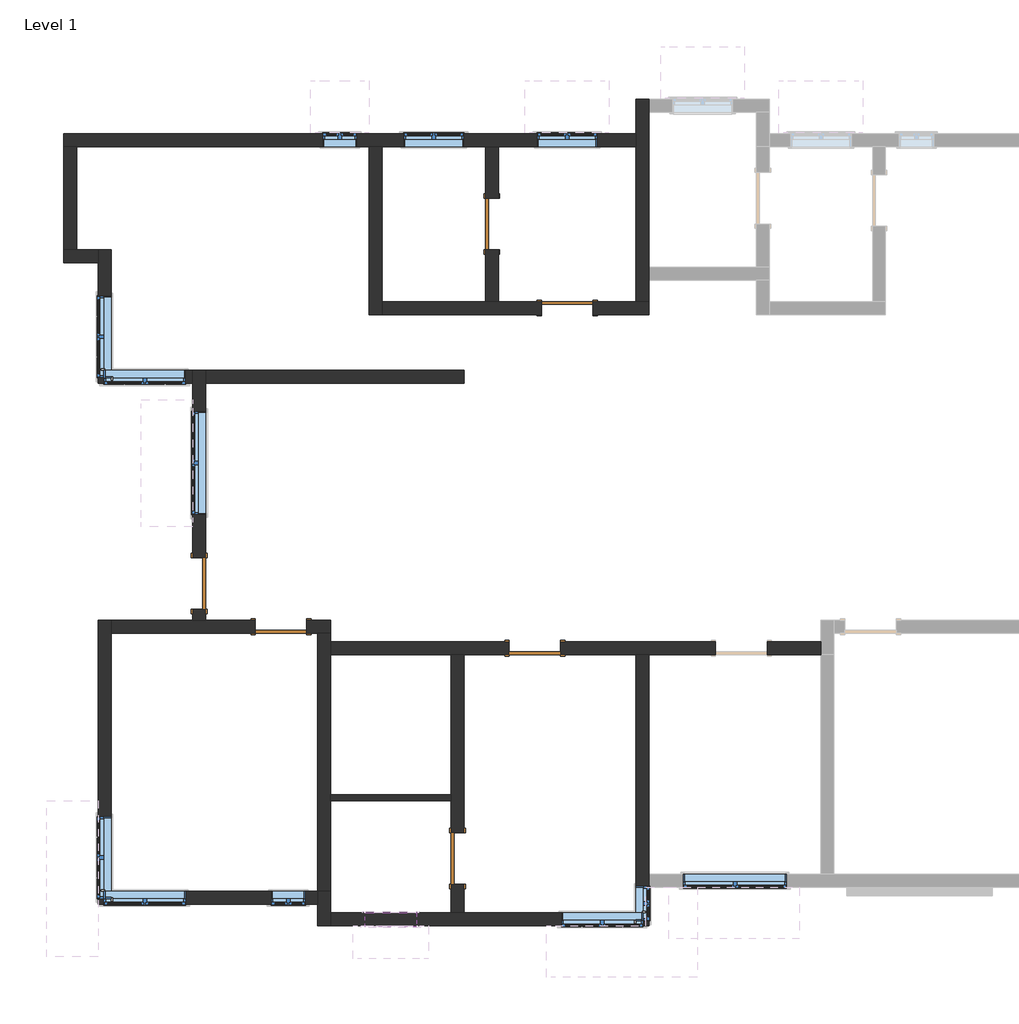
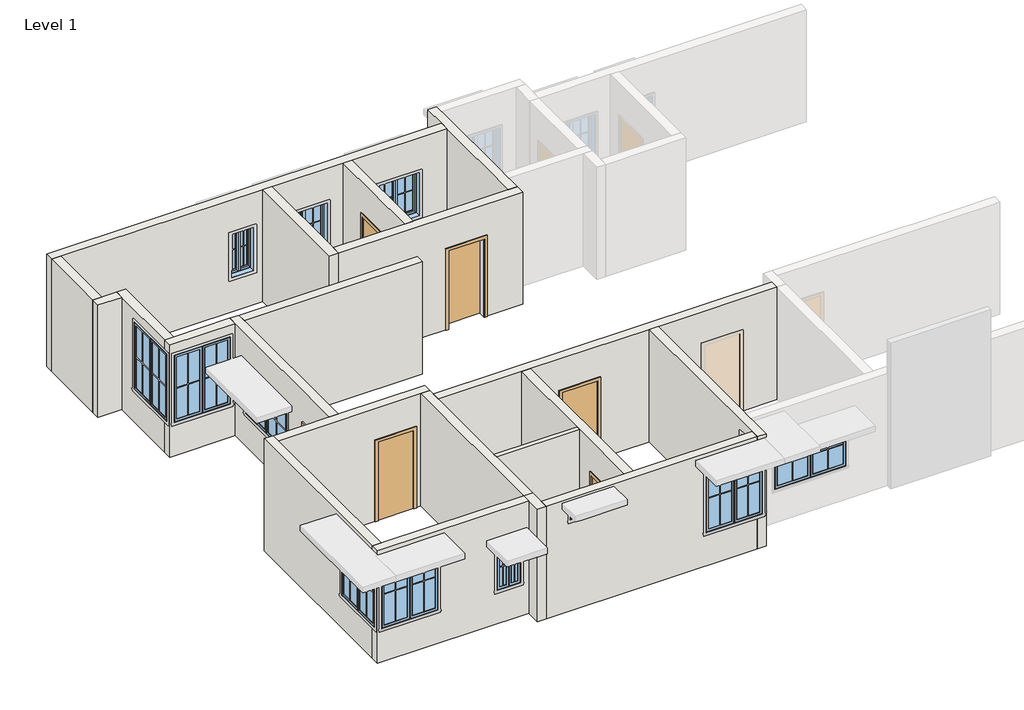
# One storey, part 1 of 3: 21 walls, 13 windows, 6 doors.
"""IFC4 building model written with IfcOpenShell, lengths in millimetres."""

from ifc_helpers import new_model, si_unit, frame, origin, origin_with_axes, place, context, project, spatial, polyline, outline, extrude, faceted_brep, transform, mapped, element, save
from components import door_0ca8825f, door_a90ba1ad, window_0389f97f, window_782a76c6, window_64f85577, window_2032b2cd, window_9ac97e1a, window_bf2f09a8

model = new_model("IFC4")

# Units and contexts
model_context = context("Model", 3, world=origin())
ifc_project = project(units=[si_unit("LENGTHUNIT", "METRE", prefix="MILLI")], contexts=[model_context])

# Site, building, storey
site = spatial("IfcSite", under=ifc_project)
building = spatial("IfcBuilding", under=site)
storey = spatial("IfcBuildingStorey", under=building, Name="Level 1", Elevation=0.0)

# Doors
placement = place(None, origin())
door_shape = door_0ca8825f(model_context)
element("IfcDoor", 1, ObjectType="Single-Flush : 36\" x 84\"", at=placement, inside=storey, context=model_context, shape_type="MappedRepresentation", body=[
    mapped(door_shape, transform((-40282.9145004, 11700.8256148, 0.0), x_axis=(0.0, -1.0, 0.0), y_axis=(1.0, 0.0, 0.0), z_axis=(0.0, 0.0, 1.0))),
])
element("IfcDoor", 2, ObjectType="Single-Flush : 36\" x 84\"", at=placement, inside=storey, context=model_context, shape_type="MappedRepresentation", body=[
    mapped(door_shape, transform((-33767.8145004, 16577.6256148, 0.0), x_axis=(1.0, 0.0, 0.0), y_axis=(0.0, 1.0, 0.0), z_axis=(0.0, 0.0, 1.0))),
])
element("IfcDoor", 3, ObjectType="Single-Flush : 36\" x 84\"", at=placement, inside=storey, context=model_context, shape_type="MappedRepresentation", body=[
    mapped(door_shape, transform((-35101.3145004, 18063.5256148, 0.0), x_axis=(0.0, 1.0, 0.0), y_axis=(-1.0, 0.0, 0.0), z_axis=(0.0, 0.0, 1.0))),
])
element("IfcDoor", 4, ObjectType="Single-Flush : 36\" x 84\"", at=placement, inside=storey, context=model_context, shape_type="MappedRepresentation", body=[
    mapped(door_shape, transform((-34339.3145004, 10557.8256148, 0.0), x_axis=(-1.0, 0.0, 0.0), y_axis=(0.0, -1.0, 0.0), z_axis=(0.0, 0.0, 1.0))),
])
element("IfcDoor", 5, ObjectType="Single-Flush : 36\" x 84\"", at=placement, inside=storey, context=model_context, shape_type="MappedRepresentation", body=[
    mapped(door_shape, transform((-35710.9145004, 6833.4722085, 0.0), x_axis=(0.0, 1.0, 0.0), y_axis=(-1.0, 0.0, 0.0), z_axis=(0.0, 0.0, 1.0))),
])
door_2_shape = door_a90ba1ad(model_context)
element("IfcDoor", 6, ObjectType="Single-Flush : 36\" x 84\"", at=placement, inside=storey, context=model_context, shape_type="MappedRepresentation", body=[
    mapped(door_2_shape, transform((-38835.1145004, 10938.8256148, 0.0), x_axis=(1.0, 0.0, 0.0), y_axis=(0.0, 1.0, 0.0), z_axis=(0.0, 0.0, 1.0))),
])

# Walls
element("IfcWall", 7, ObjectType="wall 4.5", at=placement, inside=storey, context=model_context, shape_type="SweptSolid", body=[
    extrude(outline(polyline([(-35825.2145004, 7852.6472085), (-37958.8145004, 7852.6472085), (-37958.8145004, 7966.9472085), (-35825.2145004, 7966.9472085), (-35825.2145004, 7852.6472085)])), origin_with_axes(), (0.0, 0.0, 1.0), 3048.0),
])
element("IfcWall", 8, ObjectType="wall 9\"", at=placement, inside=storey, context=model_context, shape_type="Brep", body=[
    faceted_brep([(-42683.2145004, 19435.1256148, 0.0), (-42454.6145004, 19435.1256148, 0.0), (-37273.0145004, 19435.1256148, 0.0), (-37044.4145004, 19435.1256148, 0.0), (-35215.6145004, 19435.1256148, 0.0), (-34987.0145004, 19435.1256148, 0.0), (-32548.6145004, 19435.1256148, 0.0), (-32548.6145004, 19435.1256148, 3048.0), (-34987.0145004, 19435.1256148, 3048.0), (-35215.6145004, 19435.1256148, 3048.0), (-37044.4145004, 19435.1256148, 3048.0), (-37273.0145004, 19435.1256148, 3048.0), (-42454.6145004, 19435.1256148, 3048.0), (-42683.2145004, 19435.1256148, 3048.0), (-35596.6145004, 19435.1256148, 2133.6), (-35596.6145004, 19435.1256148, 914.4), (-36663.4145004, 19435.1256148, 914.4), (-36663.4145004, 19435.1256148, 2133.6), (-33234.4145004, 19435.1256148, 2133.6), (-33234.4145004, 19435.1256148, 914.4), (-34301.2145004, 19435.1256148, 914.4), (-34301.2145004, 19435.1256148, 2133.6), (-37488.9145004, 19435.1256148, 2133.6), (-37488.9145004, 19435.1256148, 914.4), (-38098.5145004, 19435.1256148, 914.4), (-38098.5145004, 19435.1256148, 2133.6), (-42683.2145004, 19663.7256148, 0.0), (-42683.2145004, 19663.7256148, 3048.0), (-32548.6145004, 19663.7256148, 3048.0), (-32548.6145004, 19663.7256148, 0.0), (-35596.6145004, 19663.7256148, 2133.6), (-36663.4145004, 19663.7256148, 2133.6), (-36663.4145004, 19663.7256148, 914.4), (-35596.6145004, 19663.7256148, 914.4), (-33234.4145004, 19663.7256148, 2133.6), (-34301.2145004, 19663.7256148, 2133.6), (-34301.2145004, 19663.7256148, 914.4), (-33234.4145004, 19663.7256148, 914.4), (-37488.9145004, 19663.7256148, 2133.6), (-38098.5145004, 19663.7256148, 2133.6), (-38098.5145004, 19663.7256148, 914.4), (-37488.9145004, 19663.7256148, 914.4)], [[[0, 1, 2, 3, 4, 5, 6, 7, 8, 9, 10, 11, 12, 13], [14, 15, 16, 17], [18, 19, 20, 21], [22, 23, 24, 25]], [[26, 27, 28, 29], [30, 31, 32, 33], [34, 35, 36, 37], [38, 39, 40, 41]], [[6, 5, 4, 3, 2, 1, 0, 26, 29]], [[13, 12, 11, 10, 9, 8, 7, 28, 27]], [[7, 6, 29, 28]], [[0, 13, 27, 26]], [[15, 14, 30, 33]], [[16, 15, 33, 32]], [[17, 16, 32, 31]], [[14, 17, 31, 30]], [[19, 18, 34, 37]], [[20, 19, 37, 36]], [[21, 20, 36, 35]], [[18, 21, 35, 34]], [[23, 22, 38, 41]], [[24, 23, 41, 40]], [[25, 24, 40, 39]], [[22, 25, 39, 38]]]),
])
element("IfcWall", 9, ObjectType="wall 9\"", at=placement, inside=storey, context=model_context, shape_type="Brep", body=[
    faceted_brep([(-32320.0145004, 16691.9256148, 0.0), (-32320.0145004, 17072.9256148, 0.0), (-32320.0145004, 17301.5256148, 0.0), (-32320.0145004, 20044.7256148, 0.0), (-32320.0145004, 20273.3256148, 0.0), (-32320.0145004, 20273.3256148, 3048.0), (-32320.0145004, 20044.7256148, 3048.0), (-32320.0145004, 17301.5256148, 3048.0), (-32320.0145004, 17072.9256148, 3048.0), (-32320.0145004, 16691.9256148, 3048.0), (-32548.6145004, 16691.9256148, 0.0), (-32548.6145004, 16691.9256148, 3048.0), (-32548.6145004, 19435.1256148, 3048.0), (-32548.6145004, 19663.7256148, 3048.0), (-32548.6145004, 20273.3256148, 3048.0), (-32548.6145004, 20273.3256148, 0.0), (-32548.6145004, 19663.7256148, 0.0), (-32548.6145004, 19435.1256148, 0.0)], [[[0, 1, 2, 3, 4, 5, 6, 7, 8, 9]], [[10, 11, 12, 13, 14, 15, 16, 17]], [[4, 3, 2, 1, 0, 10, 17, 16, 15]], [[9, 8, 7, 6, 5, 14, 13, 12, 11]], [[5, 4, 15, 14]], [[0, 9, 11, 10]]]),
])
element("IfcWall", 10, ObjectType="wall 9\"", at=placement, inside=storey, context=model_context, shape_type="Brep", body=[
    faceted_brep([(-32548.6145004, 10443.5256148, 0.0), (-32548.6145004, 5871.4472085, 0.0), (-32548.6145004, 5642.8472085, 0.0), (-32548.6145004, 5642.8472085, 914.4), (-32548.6145004, 5871.4472085, 914.4), (-32548.6145004, 6341.3472085, 914.4), (-32548.6145004, 6341.3472085, 2743.2), (-32548.6145004, 5871.4472085, 2743.2), (-32548.6145004, 5642.8472085, 2743.2), (-32548.6145004, 5642.8472085, 3048.0), (-32548.6145004, 5871.4472085, 3048.0), (-32548.6145004, 10443.5256148, 3048.0), (-32320.0145004, 5642.8472085, 0.0), (-32320.0145004, 6328.7256148, 0.0), (-32320.0145004, 6557.3256148, 0.0), (-32320.0145004, 10443.5256148, 0.0), (-32320.0145004, 10443.5256148, 3048.0), (-32320.0145004, 6557.3256148, 3048.0), (-32320.0145004, 6328.7256148, 3048.0), (-32320.0145004, 5642.8472085, 3048.0), (-32320.0145004, 5731.7472085, 914.4), (-32320.0145004, 5731.7472085, 2743.2), (-32320.0145004, 6341.3472085, 2743.2), (-32320.0145004, 6341.3472085, 914.4), (-32421.6145004, 5642.8472085, 2743.2), (-32421.6145004, 5642.8472085, 914.4), (-32421.6145004, 5731.7472085, 914.4), (-32421.6145004, 5731.7472085, 2743.2)], [[[0, 1, 2, 3, 4, 5, 6, 7, 8, 9, 10, 11]], [[12, 13, 14, 15, 16, 17, 18, 19], [20, 21, 22, 23]], [[2, 1, 0, 15, 14, 13, 12]], [[11, 10, 9, 19, 18, 17, 16]], [[2, 12, 19, 9, 8, 24, 25, 3]], [[0, 11, 16, 15]], [[3, 25, 26, 20, 23, 5, 4]], [[25, 24, 27, 26]], [[24, 8, 7, 6, 22, 21, 27]], [[27, 21, 20, 26]], [[5, 23, 22, 6]]]),
])
element("IfcWall", 11, ObjectType="wall 9\"", at=placement, inside=storey, context=model_context, shape_type="Brep", body=[
    faceted_brep([(-32548.6145004, 5871.4472085, 0.0), (-35596.6145004, 5871.4472085, 0.0), (-35825.2145004, 5871.4472085, 0.0), (-37958.8145004, 5871.4472085, 0.0), (-37958.8145004, 5871.4472085, 3048.0), (-35825.2145004, 5871.4472085, 3048.0), (-35596.6145004, 5871.4472085, 3048.0), (-32548.6145004, 5871.4472085, 3048.0), (-32548.6145004, 5871.4472085, 2743.2), (-33869.4145004, 5871.4472085, 2743.2), (-33869.4145004, 5871.4472085, 914.4), (-32548.6145004, 5871.4472085, 914.4), (-37349.2145004, 5871.4472085, 2781.3), (-37349.2145004, 5871.4472085, 2476.5), (-36434.8145004, 5871.4472085, 2476.5), (-36434.8145004, 5871.4472085, 2781.3), (-37958.8145004, 5642.8472085, 0.0), (-32548.6145004, 5642.8472085, 0.0), (-32548.6145004, 5642.8472085, 914.4), (-33869.4145004, 5642.8472085, 914.4), (-33869.4145004, 5642.8472085, 2743.2), (-32548.6145004, 5642.8472085, 2743.2), (-32548.6145004, 5642.8472085, 3048.0), (-37958.8145004, 5642.8472085, 3048.0), (-37349.2145004, 5642.8472085, 2781.3), (-36434.8145004, 5642.8472085, 2781.3), (-36434.8145004, 5642.8472085, 2476.5), (-37349.2145004, 5642.8472085, 2476.5)], [[[0, 1, 2, 3, 4, 5, 6, 7, 8, 9, 10, 11], [12, 13, 14, 15]], [[16, 17, 18, 19, 20, 21, 22, 23], [24, 25, 26, 27]], [[3, 2, 1, 0, 17, 16]], [[7, 6, 5, 4, 23, 22]], [[7, 22, 21, 8]], [[17, 0, 11, 18]], [[4, 3, 16, 23]], [[13, 12, 24, 27]], [[14, 13, 27, 26]], [[15, 14, 26, 25]], [[12, 15, 25, 24]], [[9, 20, 19, 10]], [[10, 19, 18, 11]], [[20, 9, 8, 21]]]),
])
element("IfcWall", 12, ObjectType="wall 9\"", at=placement, inside=storey, context=model_context, shape_type="Brep", body=[
    faceted_brep([(-37958.8145004, 5642.8472085, 0.0), (-37958.8145004, 5871.4472085, 0.0), (-37958.8145004, 6252.5256148, 0.0), (-37958.8145004, 6252.5256148, 3048.0), (-37958.8145004, 5871.4472085, 3048.0), (-37958.8145004, 5642.8472085, 3048.0), (-38187.4145004, 5642.8472085, 0.0), (-38187.4145004, 5642.8472085, 3048.0), (-38187.4145004, 6023.9256148, 3048.0), (-38187.4145004, 6252.5256148, 3048.0), (-38187.4145004, 6252.5256148, 0.0), (-38187.4145004, 6023.9256148, 0.0)], [[[0, 1, 2, 3, 4, 5]], [[6, 7, 8, 9, 10, 11]], [[2, 1, 0, 6, 11, 10]], [[5, 4, 3, 9, 8, 7]], [[0, 5, 7, 6]], [[3, 2, 10, 9]]]),
])
element("IfcWall", 13, ObjectType="wall 9\"", at=placement, inside=storey, context=model_context, shape_type="Brep", body=[
    faceted_brep([(-38187.4145004, 6252.5256148, 0.0), (-41845.0145004, 6252.5256148, 0.0), (-42073.6145004, 6252.5256148, 0.0), (-42073.6145004, 6252.5256148, 914.4), (-41845.0145004, 6252.5256148, 914.4), (-40524.2145004, 6252.5256148, 914.4), (-40524.2145004, 6252.5256148, 2743.2), (-41845.0145004, 6252.5256148, 2743.2), (-42073.6145004, 6252.5256148, 2743.2), (-42073.6145004, 6252.5256148, 3048.0), (-41845.0145004, 6252.5256148, 3048.0), (-38187.4145004, 6252.5256148, 3048.0), (-39012.9145004, 6252.5256148, 2133.6), (-39012.9145004, 6252.5256148, 914.4), (-38403.3145004, 6252.5256148, 914.4), (-38403.3145004, 6252.5256148, 2133.6), (-42073.6145004, 6023.9256148, 0.0), (-38187.4145004, 6023.9256148, 0.0), (-38187.4145004, 6023.9256148, 3048.0), (-42073.6145004, 6023.9256148, 3048.0), (-39012.9145004, 6023.9256148, 914.4), (-39012.9145004, 6023.9256148, 2133.6), (-38403.3145004, 6023.9256148, 2133.6), (-38403.3145004, 6023.9256148, 914.4), (-41972.0145004, 6023.9256148, 914.4), (-41972.0145004, 6023.9256148, 2743.2), (-40524.2145004, 6023.9256148, 2743.2), (-40524.2145004, 6023.9256148, 914.4), (-42073.6145004, 6125.5256148, 2743.2), (-42073.6145004, 6125.5256148, 914.4), (-41972.0145004, 6125.5256148, 914.4), (-41972.0145004, 6125.5256148, 2743.2)], [[[0, 1, 2, 3, 4, 5, 6, 7, 8, 9, 10, 11], [12, 13, 14, 15]], [[16, 17, 18, 19], [20, 21, 22, 23], [24, 25, 26, 27]], [[2, 1, 0, 17, 16]], [[11, 10, 9, 19, 18]], [[0, 11, 18, 17]], [[2, 16, 19, 9, 8, 28, 29, 3]], [[13, 12, 21, 20]], [[14, 13, 20, 23]], [[15, 14, 23, 22]], [[12, 15, 22, 21]], [[25, 24, 30, 31]], [[24, 27, 5, 4, 3, 29, 30]], [[6, 5, 27, 26]], [[26, 25, 31, 28, 8, 7, 6]], [[28, 31, 30, 29]]]),
])
element("IfcWall", 14, ObjectType="wall 9\"", at=placement, inside=storey, context=model_context, shape_type="Brep", body=[
    faceted_brep([(-41845.0145004, 6252.5256148, 0.0), (-41845.0145004, 10824.5256148, 0.0), (-41845.0145004, 11053.1256148, 0.0), (-41845.0145004, 11053.1256148, 3048.0), (-41845.0145004, 10824.5256148, 3048.0), (-41845.0145004, 6252.5256148, 3048.0), (-41845.0145004, 6252.5256148, 2743.2), (-41845.0145004, 7573.3256148, 2743.2), (-41845.0145004, 7573.3256148, 914.4), (-41845.0145004, 6252.5256148, 914.4), (-42073.6145004, 11053.1256148, 0.0), (-42073.6145004, 6252.5256148, 0.0), (-42073.6145004, 6252.5256148, 914.4), (-42073.6145004, 7573.3256148, 914.4), (-42073.6145004, 7573.3256148, 2743.2), (-42073.6145004, 6252.5256148, 2743.2), (-42073.6145004, 6252.5256148, 3048.0), (-42073.6145004, 11053.1256148, 3048.0), (-41972.0145004, 6252.5256148, 2743.2), (-41972.0145004, 6252.5256148, 914.4)], [[[0, 1, 2, 3, 4, 5, 6, 7, 8, 9]], [[10, 11, 12, 13, 14, 15, 16, 17]], [[2, 1, 0, 11, 10]], [[5, 4, 3, 17, 16]], [[5, 16, 15, 18, 6]], [[11, 0, 9, 19, 12]], [[3, 2, 10, 17]], [[7, 14, 13, 8]], [[8, 13, 12, 19, 9]], [[14, 7, 6, 18, 15]]]),
])
element("IfcWall", 15, ObjectType="wall 9\"", at=placement, inside=storey, context=model_context, shape_type="Brep", body=[
    faceted_brep([(-38377.9145004, 10824.5256148, 2133.6), (-38377.9145004, 10824.5256148, 0.0), (-38187.4145004, 10824.5256148, 0.0), (-37958.8145004, 10824.5256148, 0.0), (-37958.8145004, 10824.5256148, 3048.0), (-38187.4145004, 10824.5256148, 3048.0), (-41845.0145004, 10824.5256148, 3048.0), (-41845.0145004, 10824.5256148, 0.0), (-39292.3145004, 10824.5256148, 0.0), (-39292.3145004, 10824.5256148, 2133.6), (-37958.8145004, 11053.1256148, 0.0), (-38377.9145004, 11053.1256148, 0.0), (-38377.9145004, 11053.1256148, 2133.6), (-39292.3145004, 11053.1256148, 2133.6), (-39292.3145004, 11053.1256148, 0.0), (-40168.6145004, 11053.1256148, 0.0), (-40397.2145004, 11053.1256148, 0.0), (-41845.0145004, 11053.1256148, 0.0), (-41845.0145004, 11053.1256148, 3048.0), (-40397.2145004, 11053.1256148, 3048.0), (-40168.6145004, 11053.1256148, 3048.0), (-37958.8145004, 11053.1256148, 3048.0)], [[[0, 1, 2, 3, 4, 5, 6, 7, 8, 9]], [[10, 11, 12, 13, 14, 15, 16, 17, 18, 19, 20, 21]], [[8, 7, 17, 16, 15, 14]], [[3, 2, 1, 11, 10]], [[6, 5, 4, 21, 20, 19, 18]], [[7, 6, 18, 17]], [[4, 3, 10, 21]], [[12, 11, 1, 0]], [[13, 12, 0, 9]], [[14, 13, 9, 8]]]),
])
element("IfcWall", 16, ObjectType="wall 9\"", at=placement, inside=storey, context=model_context, shape_type="Brep", body=[
    faceted_brep([(-40168.6145004, 11053.1256148, 0.0), (-40168.6145004, 11243.6256148, 0.0), (-40168.6145004, 11243.6256148, 2133.6), (-40168.6145004, 12158.0256148, 2133.6), (-40168.6145004, 12158.0256148, 0.0), (-40168.6145004, 15244.1256148, 0.0), (-40168.6145004, 15472.7256148, 0.0), (-40168.6145004, 15472.7256148, 3048.0), (-40168.6145004, 15244.1256148, 3048.0), (-40168.6145004, 11053.1256148, 3048.0), (-40168.6145004, 14748.8256148, 2133.6), (-40168.6145004, 14748.8256148, 914.4), (-40168.6145004, 12920.0256148, 914.4), (-40168.6145004, 12920.0256148, 2133.6), (-40397.2145004, 11243.6256148, 2133.6), (-40397.2145004, 11243.6256148, 0.0), (-40397.2145004, 11053.1256148, 0.0), (-40397.2145004, 11053.1256148, 3048.0), (-40397.2145004, 15244.1256148, 3048.0), (-40397.2145004, 15472.7256148, 3048.0), (-40397.2145004, 15472.7256148, 0.0), (-40397.2145004, 15244.1256148, 0.0), (-40397.2145004, 12158.0256148, 0.0), (-40397.2145004, 12158.0256148, 2133.6), (-40397.2145004, 14748.8256148, 2133.6), (-40397.2145004, 12920.0256148, 2133.6), (-40397.2145004, 12920.0256148, 914.4), (-40397.2145004, 14748.8256148, 914.4)], [[[0, 1, 2, 3, 4, 5, 6, 7, 8, 9], [10, 11, 12, 13]], [[14, 15, 16, 17, 18, 19, 20, 21, 22, 23], [24, 25, 26, 27]], [[16, 15, 1, 0]], [[22, 21, 20, 6, 5, 4]], [[9, 8, 7, 19, 18, 17]], [[0, 9, 17, 16]], [[7, 6, 20, 19]], [[2, 1, 15, 14]], [[3, 2, 14, 23]], [[4, 3, 23, 22]], [[11, 10, 24, 27]], [[12, 11, 27, 26]], [[13, 12, 26, 25]], [[10, 13, 25, 24]]]),
])
element("IfcWall", 17, ObjectType="wall 9\"", at=placement, inside=storey, context=model_context, shape_type="Brep", body=[
    faceted_brep([(-40397.2145004, 15472.7256148, 0.0), (-41845.0145004, 15472.7256148, 0.0), (-42073.6145004, 15472.7256148, 0.0), (-42073.6145004, 15472.7256148, 914.4), (-41845.0145004, 15472.7256148, 914.4), (-40524.2145004, 15472.7256148, 914.4), (-40524.2145004, 15472.7256148, 2743.2), (-41845.0145004, 15472.7256148, 2743.2), (-42073.6145004, 15472.7256148, 2743.2), (-42073.6145004, 15472.7256148, 3048.0), (-41845.0145004, 15472.7256148, 3048.0), (-40397.2145004, 15472.7256148, 3048.0), (-42073.6145004, 15244.1256148, 0.0), (-40397.2145004, 15244.1256148, 0.0), (-40397.2145004, 15244.1256148, 3048.0), (-42073.6145004, 15244.1256148, 3048.0), (-41972.0145004, 15244.1256148, 914.4), (-41972.0145004, 15244.1256148, 2743.2), (-40524.2145004, 15244.1256148, 2743.2), (-40524.2145004, 15244.1256148, 914.4), (-42073.6145004, 15345.7256148, 2743.2), (-42073.6145004, 15345.7256148, 914.4), (-41972.0145004, 15345.7256148, 914.4), (-41972.0145004, 15345.7256148, 2743.2)], [[[0, 1, 2, 3, 4, 5, 6, 7, 8, 9, 10, 11]], [[12, 13, 14, 15], [16, 17, 18, 19]], [[2, 1, 0, 13, 12]], [[11, 10, 9, 15, 14]], [[0, 11, 14, 13]], [[2, 12, 15, 9, 8, 20, 21, 3]], [[17, 16, 22, 23]], [[16, 19, 5, 4, 3, 21, 22]], [[6, 5, 19, 18]], [[18, 17, 23, 20, 8, 7, 6]], [[20, 23, 22, 21]]]),
])
element("IfcWall", 18, ObjectType="wall 9\"", at=placement, inside=storey, context=model_context, shape_type="Brep", body=[
    faceted_brep([(-41845.0145004, 15472.7256148, 0.0), (-41845.0145004, 17606.3256148, 0.0), (-41845.0145004, 17606.3256148, 3048.0), (-41845.0145004, 15472.7256148, 3048.0), (-41845.0145004, 15472.7256148, 2743.2), (-41845.0145004, 16793.5256148, 2743.2), (-41845.0145004, 16793.5256148, 914.4), (-41845.0145004, 15472.7256148, 914.4), (-42073.6145004, 17606.3256148, 0.0), (-42073.6145004, 17377.7256148, 0.0), (-42073.6145004, 15472.7256148, 0.0), (-42073.6145004, 15472.7256148, 914.4), (-42073.6145004, 16793.5256148, 914.4), (-42073.6145004, 16793.5256148, 2743.2), (-42073.6145004, 15472.7256148, 2743.2), (-42073.6145004, 15472.7256148, 3048.0), (-42073.6145004, 17377.7256148, 3048.0), (-42073.6145004, 17606.3256148, 3048.0), (-41972.0145004, 15472.7256148, 2743.2), (-41972.0145004, 15472.7256148, 914.4)], [[[0, 1, 2, 3, 4, 5, 6, 7]], [[8, 9, 10, 11, 12, 13, 14, 15, 16, 17]], [[1, 0, 10, 9, 8]], [[3, 2, 17, 16, 15]], [[3, 15, 14, 18, 4]], [[10, 0, 7, 19, 11]], [[2, 1, 8, 17]], [[5, 13, 12, 6]], [[6, 12, 11, 19, 7]], [[13, 5, 4, 18, 14]]]),
])
element("IfcWall", 19, ObjectType="wall 9\"", at=placement, inside=storey, context=model_context, shape_type="Brep", body=[
    faceted_brep([(-42073.6145004, 17606.3256148, 0.0), (-42454.6145004, 17606.3256148, 0.0), (-42683.2145004, 17606.3256148, 0.0), (-42683.2145004, 17606.3256148, 3048.0), (-42454.6145004, 17606.3256148, 3048.0), (-42073.6145004, 17606.3256148, 3048.0), (-42073.6145004, 17377.7256148, 0.0), (-42073.6145004, 17377.7256148, 3048.0), (-42683.2145004, 17377.7256148, 3048.0), (-42683.2145004, 17377.7256148, 0.0)], [[[0, 1, 2, 3, 4, 5]], [[6, 7, 8, 9]], [[2, 1, 0, 6, 9]], [[5, 4, 3, 8, 7]], [[0, 5, 7, 6]], [[3, 2, 9, 8]]]),
])
element("IfcWall", 20, ObjectType="wall 9\"", at=placement, inside=storey, context=model_context, shape_type="SweptSolid", body=[
    extrude(outline(polyline([(-42454.6145004, 19435.1256148), (-42454.6145004, 17606.3256148), (-42683.2145004, 17606.3256148), (-42683.2145004, 19435.1256148), (-42454.6145004, 19435.1256148)])), origin_with_axes(), (0.0, 0.0, 1.0), 3048.0),
])
element("IfcWall", 21, ObjectType="wall 9\"", at=placement, inside=storey, context=model_context, shape_type="Brep", body=[
    faceted_brep([(-37273.0145004, 19435.1256148, 0.0), (-37273.0145004, 16463.3256148, 0.0), (-37273.0145004, 16463.3256148, 3048.0), (-37273.0145004, 19435.1256148, 3048.0), (-37044.4145004, 19435.1256148, 0.0), (-37044.4145004, 19435.1256148, 3048.0), (-37044.4145004, 16691.9256148, 3048.0), (-37044.4145004, 16463.3256148, 3048.0), (-37044.4145004, 16463.3256148, 0.0), (-37044.4145004, 16691.9256148, 0.0)], [[[0, 1, 2, 3]], [[4, 5, 6, 7, 8, 9]], [[1, 0, 4, 9, 8]], [[3, 2, 7, 6, 5]], [[0, 3, 5, 4]], [[2, 1, 8, 7]]]),
])
element("IfcWall", 22, ObjectType="wall 9\"", at=placement, inside=storey, context=model_context, shape_type="Brep", body=[
    faceted_brep([(-33310.6145004, 16463.3256148, 2133.6), (-33310.6145004, 16463.3256148, 0.0), (-32320.0145004, 16463.3256148, 0.0), (-32320.0145004, 16463.3256148, 3048.0), (-37044.4145004, 16463.3256148, 3048.0), (-37044.4145004, 16463.3256148, 0.0), (-34225.0145004, 16463.3256148, 0.0), (-34225.0145004, 16463.3256148, 2133.6), (-32320.0145004, 16691.9256148, 0.0), (-32548.6145004, 16691.9256148, 0.0), (-33310.6145004, 16691.9256148, 0.0), (-33310.6145004, 16691.9256148, 2133.6), (-34225.0145004, 16691.9256148, 2133.6), (-34225.0145004, 16691.9256148, 0.0), (-34987.0145004, 16691.9256148, 0.0), (-35215.6145004, 16691.9256148, 0.0), (-37044.4145004, 16691.9256148, 0.0), (-37044.4145004, 16691.9256148, 3048.0), (-35215.6145004, 16691.9256148, 3048.0), (-34987.0145004, 16691.9256148, 3048.0), (-32548.6145004, 16691.9256148, 3048.0), (-32320.0145004, 16691.9256148, 3048.0)], [[[0, 1, 2, 3, 4, 5, 6, 7]], [[8, 9, 10, 11, 12, 13, 14, 15, 16, 17, 18, 19, 20, 21]], [[6, 5, 16, 15, 14, 13]], [[2, 1, 10, 9, 8]], [[4, 3, 21, 20, 19, 18, 17]], [[5, 4, 17, 16]], [[3, 2, 8, 21]], [[11, 10, 1, 0]], [[12, 11, 0, 7]], [[13, 12, 7, 6]]]),
])
element("IfcWall", 23, ObjectType="wall 9\"", at=placement, inside=storey, context=model_context, shape_type="SweptSolid", body=[
    extrude(outline(polyline([(19435.1256148, 0.0), (18520.7256148, 0.0), (18520.7256148, 2133.6), (17606.3256148, 2133.6), (17606.3256148, 0.0), (16691.9256148, 0.0), (16691.9256148, 3048.0), (19435.1256148, 3048.0), (19435.1256148, 0.0)])), frame((-35215.6145004, 0.0, 0.0), z_axis=(1.0, 0.0, 0.0), x_axis=(0.0, 1.0, 0.0)), (0.0, 0.0, 1.0), 228.6),
])
element("IfcWall", 24, ObjectType="wall 9\"", at=placement, inside=storey, context=model_context, shape_type="SweptSolid", body=[
    extrude(outline(polyline([(-35596.6145004, 15244.1256148), (-40168.6145004, 15244.1256148), (-40168.6145004, 15472.7256148), (-35596.6145004, 15472.7256148), (-35596.6145004, 15244.1256148)])), origin_with_axes(), (0.0, 0.0, 1.0), 3048.0),
])
element("IfcWall", 25, ObjectType="wall 9\"", at=placement, inside=storey, context=model_context, shape_type="Brep", body=[
    faceted_brep([(-38187.4145004, 10824.5256148, 0.0), (-38187.4145004, 6252.5256148, 0.0), (-38187.4145004, 6252.5256148, 3048.0), (-38187.4145004, 10824.5256148, 3048.0), (-37958.8145004, 10824.5256148, 0.0), (-37958.8145004, 10824.5256148, 3048.0), (-37958.8145004, 10672.1256148, 3048.0), (-37958.8145004, 10443.5256148, 3048.0), (-37958.8145004, 7966.9472085, 3048.0), (-37958.8145004, 7852.6472085, 3048.0), (-37958.8145004, 6252.5256148, 3048.0), (-37958.8145004, 6252.5256148, 0.0), (-37958.8145004, 7852.6472085, 0.0), (-37958.8145004, 7966.9472085, 0.0), (-37958.8145004, 10443.5256148, 0.0), (-37958.8145004, 10672.1256148, 0.0)], [[[0, 1, 2, 3]], [[4, 5, 6, 7, 8, 9, 10, 11, 12, 13, 14, 15]], [[1, 0, 4, 15, 14, 13, 12, 11]], [[3, 2, 10, 9, 8, 7, 6, 5]], [[0, 3, 5, 4]], [[2, 1, 11, 10]]]),
])
element("IfcWall", 26, ObjectType="wall 9\"", at=placement, inside=storey, context=model_context, shape_type="Brep", body=[
    faceted_brep([(-37958.8145004, 10443.5256148, 0.0), (-35825.2145004, 10443.5256148, 0.0), (-35596.6145004, 10443.5256148, 0.0), (-34796.5145004, 10443.5256148, 0.0), (-34796.5145004, 10443.5256148, 2133.6), (-33882.1145004, 10443.5256148, 2133.6), (-33882.1145004, 10443.5256148, 0.0), (-32548.6145004, 10443.5256148, 0.0), (-32320.0145004, 10443.5256148, 0.0), (-31138.9145004, 10443.5256148, 0.0), (-31138.9145004, 10443.5256148, 2133.6), (-30224.5145004, 10443.5256148, 2133.6), (-30224.5145004, 10443.5256148, 0.0), (-29272.0145004, 10443.5256148, 0.0), (-29272.0145004, 10443.5256148, 3048.0), (-32320.0145004, 10443.5256148, 3048.0), (-32548.6145004, 10443.5256148, 3048.0), (-35596.6145004, 10443.5256148, 3048.0), (-35825.2145004, 10443.5256148, 3048.0), (-37958.8145004, 10443.5256148, 3048.0), (-34796.5145004, 10672.1256148, 2133.6), (-34796.5145004, 10672.1256148, 0.0), (-37958.8145004, 10672.1256148, 0.0), (-37958.8145004, 10672.1256148, 3048.0), (-29272.0145004, 10672.1256148, 3048.0), (-29272.0145004, 10672.1256148, 0.0), (-30224.5145004, 10672.1256148, 0.0), (-30224.5145004, 10672.1256148, 2133.6), (-31138.9145004, 10672.1256148, 2133.6), (-31138.9145004, 10672.1256148, 0.0), (-33882.1145004, 10672.1256148, 0.0), (-33882.1145004, 10672.1256148, 2133.6)], [[[0, 1, 2, 3, 4, 5, 6, 7, 8, 9, 10, 11, 12, 13, 14, 15, 16, 17, 18, 19]], [[20, 21, 22, 23, 24, 25, 26, 27, 28, 29, 30, 31]], [[26, 25, 13, 12]], [[30, 29, 9, 8, 7, 6]], [[22, 21, 3, 2, 1, 0]], [[19, 18, 17, 16, 15, 14, 24, 23]], [[0, 19, 23, 22]], [[14, 13, 25, 24]], [[10, 9, 29, 28]], [[11, 10, 28, 27]], [[12, 11, 27, 26]], [[4, 3, 21, 20]], [[5, 4, 20, 31]], [[6, 5, 31, 30]]]),
])
element("IfcWall", 27, ObjectType="wall 9\"", at=placement, inside=storey, context=model_context, shape_type="Brep", body=[
    faceted_brep([(-35825.2145004, 10443.5256148, 0.0), (-35825.2145004, 7966.9472085, 0.0), (-35825.2145004, 7852.6472085, 0.0), (-35825.2145004, 7290.6722085, 0.0), (-35825.2145004, 7290.6722085, 2133.6), (-35825.2145004, 6376.2722085, 2133.6), (-35825.2145004, 6376.2722085, 0.0), (-35825.2145004, 5871.4472085, 0.0), (-35825.2145004, 5871.4472085, 3048.0), (-35825.2145004, 7852.6472085, 3048.0), (-35825.2145004, 7966.9472085, 3048.0), (-35825.2145004, 10443.5256148, 3048.0), (-35596.6145004, 7290.6722085, 2133.6), (-35596.6145004, 7290.6722085, 0.0), (-35596.6145004, 10443.5256148, 0.0), (-35596.6145004, 10443.5256148, 3048.0), (-35596.6145004, 5871.4472085, 3048.0), (-35596.6145004, 5871.4472085, 0.0), (-35596.6145004, 6376.2722085, 0.0), (-35596.6145004, 6376.2722085, 2133.6)], [[[0, 1, 2, 3, 4, 5, 6, 7, 8, 9, 10, 11]], [[12, 13, 14, 15, 16, 17, 18, 19]], [[18, 17, 7, 6]], [[14, 13, 3, 2, 1, 0]], [[11, 10, 9, 8, 16, 15]], [[8, 7, 17, 16]], [[0, 11, 15, 14]], [[4, 3, 13, 12]], [[5, 4, 12, 19]], [[6, 5, 19, 18]]]),
])

# Windows
window_shape = window_0389f97f(model_context)
element("IfcWindow", 28, ObjectType="Window-Casement-Double : 24\" x 72\" 2", at=placement, inside=storey, context=model_context, shape_type="MappedRepresentation", body=[
    mapped(window_shape, transform((-32434.3145004, 6036.5472085, 0.0), x_axis=(0.0, -1.0, 0.0), y_axis=(1.0, 0.0, 0.0), z_axis=(0.0, 0.0, 1.0))),
])
window_2_shape = window_782a76c6(model_context)
element("IfcWindow", 29, ObjectType="Window-Casement-Double : 24\"X48\"", at=placement, inside=storey, context=model_context, shape_type="MappedRepresentation", body=[
    mapped(window_2_shape, transform((-38708.1145004, 6138.2256148, 0.0), x_axis=(-1.0, 0.0, 0.0), y_axis=(0.0, -1.0, 0.0), z_axis=(0.0, 0.0, 1.0))),
])
element("IfcWindow", 30, ObjectType="Window-Casement-Double : 24\"X48\"", at=placement, inside=storey, context=model_context, shape_type="MappedRepresentation", body=[
    mapped(window_2_shape, transform((-37793.7145004, 19549.4256148, 0.0), x_axis=(1.0, 0.0, 0.0), y_axis=(0.0, 1.0, 0.0), z_axis=(0.0, 0.0, 1.0))),
])
window_3_shape = window_64f85577(model_context)
element("IfcWindow", 31, ObjectType="Window-Casement-Double : 36\"X12\"", at=placement, inside=storey, context=model_context, shape_type="MappedRepresentation", body=[
    mapped(window_3_shape, transform((-36892.0145004, 5757.1472085, 1562.1), x_axis=(-1.0, 0.0, 0.0), y_axis=(0.0, -1.0, 0.0), z_axis=(0.0, 0.0, 1.0))),
])
window_4_shape = window_2032b2cd(model_context)
element("IfcWindow", 32, ObjectType="Window-Casement-Double : 42\"X48\"", at=placement, inside=storey, context=model_context, shape_type="MappedRepresentation", body=[
    mapped(window_4_shape, transform((-36130.0145004, 19549.4256148, 0.0), x_axis=(1.0, 0.0, 0.0), y_axis=(0.0, 1.0, 0.0), z_axis=(0.0, 0.0, 1.0))),
])
element("IfcWindow", 33, ObjectType="Window-Casement-Double : 42\"X48\"", at=placement, inside=storey, context=model_context, shape_type="MappedRepresentation", body=[
    mapped(window_4_shape, transform((-33767.8145004, 19549.4256148, 0.0), x_axis=(1.0, 0.0, 0.0), y_axis=(0.0, 1.0, 0.0), z_axis=(0.0, 0.0, 1.0))),
])
window_5_shape = window_9ac97e1a(model_context)
element("IfcWindow", 34, ObjectType="Window-Casement-Double : 57\" x 72\"", at=placement, inside=storey, context=model_context, shape_type="MappedRepresentation", body=[
    mapped(window_5_shape, transform((-33145.5145004, 5757.1472085, 0.0), x_axis=(-1.0, 0.0, 0.0), y_axis=(0.0, -1.0, 0.0), z_axis=(0.0, 0.0, 1.0))),
])
element("IfcWindow", 35, ObjectType="Window-Casement-Double : 57\" x 72\"", at=placement, inside=storey, context=model_context, shape_type="MappedRepresentation", body=[
    mapped(window_5_shape, transform((-41248.1145004, 15358.4256148, 0.0), x_axis=(-1.0, 0.0, 0.0), y_axis=(0.0, -1.0, 0.0), z_axis=(0.0, 0.0, 1.0))),
])
element("IfcWindow", 36, ObjectType="Window-Casement-Double : 57\" x 72\"", at=placement, inside=storey, context=model_context, shape_type="MappedRepresentation", body=[
    mapped(window_5_shape, transform((-41959.3145004, 16069.6256148, 0.0), x_axis=(0.0, 1.0, 0.0), y_axis=(-1.0, 0.0, 0.0), z_axis=(0.0, 0.0, 1.0))),
])
element("IfcWindow", 37, ObjectType="Window-Casement-Double : 57\" x 72\"", at=placement, inside=storey, context=model_context, shape_type="MappedRepresentation", body=[
    mapped(window_5_shape, transform((-41248.1145004, 6138.2256148, 0.0), x_axis=(-1.0, 0.0, 0.0), y_axis=(0.0, -1.0, 0.0), z_axis=(0.0, 0.0, 1.0))),
])
element("IfcWindow", 38, ObjectType="Window-Casement-Double : 57\" x 72\"", at=placement, inside=storey, context=model_context, shape_type="MappedRepresentation", body=[
    mapped(window_5_shape, transform((-41959.3145004, 6849.4256148, 0.0), x_axis=(0.0, 1.0, 0.0), y_axis=(-1.0, 0.0, 0.0), z_axis=(0.0, 0.0, 1.0))),
])
window_6_shape = window_bf2f09a8(model_context)
element("IfcWindow", 39, ObjectType="Window-Casement-Double : 72\"X48\" 2", at=placement, inside=storey, context=model_context, shape_type="MappedRepresentation", body=[
    mapped(window_6_shape, transform((-30796.0145004, 6443.0256148, 0.0), x_axis=(-1.0, 0.0, 0.0), y_axis=(0.0, -1.0, 0.0), z_axis=(0.0, 0.0, 1.0))),
])
element("IfcWindow", 40, ObjectType="Window-Casement-Double : 72\"X48\" 2", at=placement, inside=storey, context=model_context, shape_type="MappedRepresentation", body=[
    mapped(window_6_shape, transform((-40282.9145004, 13834.4256148, 0.0), x_axis=(0.0, 1.0, 0.0), y_axis=(-1.0, 0.0, 0.0), z_axis=(0.0, 0.0, 1.0))),
])

save(model, "model.ifc")

# Revit data of these elements
# Type "Single-Flush : 36\" x 84\""
#   Type Mark = "1"
#   Construction Type Id = "MDOOR"
#   Assembly Code = "C1020"
#   Analytic Construction = "Metal"
#   Thickness = 0' - 2"
#   Heat Transfer Coefficient (U) = 0.651978 BTU/(h·ft²·°F)
#   Height = 7' - 0"
#   Trim Projection Ext = 0' - 1"
#   Trim Projection Int = 0' - 1"
#   Trim Width = 0' - 3"
#   Width = 3' - 0"
#   Define Thermal Properties by = 1
#   Define Thermal Properties by = 1
#   Door Material = Door - Panel
#   Frame Material = Door - Frame
#   Visual Light Transmittance = 0
#   Solar Heat Gain Coefficient = 0
#   Function = (empty or 0)
#   Wall Closure = (empty or 0)
# Type "wall 4.5"
#   Assembly Code = "B2010"
#   Layers, outside or top first: 0' - 4 1/2" no material (function 1)
# Type "wall 9\""
#   Assembly Code = "B2010"
#   Layers, outside or top first: 0' - 9" no material (function 1)
# Type "Window-Casement-Double : 24\" x 72\" 2"
#   Type Mark = "28"
#   Fire Rating = "0.5h"
#   Assembly Code = "B2020100"
#   Analytic Construction = "Double glazing - domestic"
#   Frame Extension [instance default] = 0' - 0 1/4"
#   Window Inset [instance default] = 0' - 0"
#   Wall Thickness [instance default] = 0' - 6"
#   Interior Wall Closure [instance default] = 0' - 2 1/4"
#   Half Width = 1' - 0"
#   Visual Light Transmittance = 0.81
#   Thermal Resistance (R) = 1.8146 (h·ft²·°F)/BTU
#   Solar Heat Gain Coefficient = 0.76
#   Rough Width = 2' - 0 1/2"
#   Rough Height = 6' - 0 1/2"
#   Height = 6' - 0"
#   Heat Transfer Coefficient (U) = 0.5511 BTU/(h·ft²·°F)
#   Exterior Wall Closure [instance default] = 0' - 1 1/4"
#   Extension Jamb [instance default] = 0' - 2 1/4"
#   Default Sill Height = 3' - 0"
#   Width = 2' - 0"
#   Muntin Visibility = yes
#   Interior Trim Visibility [instance default] = yes
#   Exterior Trim Visibility [instance default] = yes
#   Extension Jamb Visibility [instance default] = yes
#   Interior Trim Material = Wood - Stained
#   Muntin Pattern = Muntin Pattern_2x2 : Muntin Pattern_2x2
#   Interior Trim = Trim-Window-Interior-Flat : Picture Frame
#   Interior Frame Material = Wood - Stained
#   Glass Panel Material = Glass
#   Exterior Trim Material = Clad - White
#   Exterior Trim = Trim-Window-Exterior-Flat : with Sill
#   Exterior Frame Material = Clad - White
#   Wall Closure = (empty or 0)
# Type "Window-Casement-Double : 24\"X48\""
#   Type Mark = "22"
#   Fire Rating = "0.5h"
#   Assembly Code = "B2020100"
#   Analytic Construction = "Double glazing - domestic"
#   Frame Extension [instance default] = 0' - 0 1/4"
#   Window Inset [instance default] = 0' - 0"
#   Wall Thickness [instance default] = 0' - 6"
#   Interior Wall Closure [instance default] = 0' - 2 1/4"
#   Half Width = 1' - 0"
#   Visual Light Transmittance = 0.81
#   Thermal Resistance (R) = 1.8146 (h·ft²·°F)/BTU
#   Solar Heat Gain Coefficient = 0.76
#   Rough Width = 2' - 0 1/2"
#   Rough Height = 4' - 0 1/2"
#   Height = 4' - 0"
#   Heat Transfer Coefficient (U) = 0.5511 BTU/(h·ft²·°F)
#   Exterior Wall Closure [instance default] = 0' - 1 1/4"
#   Extension Jamb [instance default] = 0' - 2 1/4"
#   Default Sill Height = 3' - 0"
#   Width = 2' - 0"
#   Muntin Visibility = yes
#   Interior Trim Visibility [instance default] = yes
#   Exterior Trim Visibility [instance default] = yes
#   Extension Jamb Visibility [instance default] = yes
#   Interior Trim Material = Wood - Stained
#   Muntin Pattern = Muntin Pattern_2x2 : Muntin Pattern_2x2
#   Interior Trim = Trim-Window-Interior-Flat : Picture Frame
#   Interior Frame Material = Wood - Stained
#   Glass Panel Material = Glass
#   Exterior Trim Material = Clad - White
#   Exterior Trim = Trim-Window-Exterior-Flat : with Sill
#   Exterior Frame Material = Clad - White
#   Wall Closure = (empty or 0)
# Type "Window-Casement-Double : 36\"X12\""
#   Type Mark = "24"
#   Fire Rating = "0.5h"
#   Assembly Code = "B2020100"
#   Analytic Construction = "Double glazing - domestic"
#   Frame Extension [instance default] = 0' - 0 1/4"
#   Window Inset [instance default] = 0' - 0"
#   Wall Thickness [instance default] = 0' - 6"
#   Interior Wall Closure [instance default] = 0' - 2 1/4"
#   Half Width = 1' - 6"
#   Visual Light Transmittance = 0.81
#   Thermal Resistance (R) = 1.8146 (h·ft²·°F)/BTU
#   Solar Heat Gain Coefficient = 0.76
#   Rough Width = 3' - 0 1/2"
#   Rough Height = 1' - 0 1/2"
#   Height = 1' - 0"
#   Heat Transfer Coefficient (U) = 0.5511 BTU/(h·ft²·°F)
#   Exterior Wall Closure [instance default] = 0' - 1 1/4"
#   Extension Jamb [instance default] = 0' - 2 1/4"
#   Default Sill Height = 3' - 0"
#   Width = 3' - 0"
#   Muntin Visibility = yes
#   Interior Trim Visibility [instance default] = yes
#   Exterior Trim Visibility [instance default] = yes
#   Extension Jamb Visibility [instance default] = yes
#   Interior Trim Material = Wood - Stained
#   Muntin Pattern = Muntin Pattern_2x2 : Muntin Pattern_2x2
#   Interior Trim = Trim-Window-Interior-Flat : Picture Frame
#   Interior Frame Material = Wood - Stained
#   Glass Panel Material = Glass
#   Exterior Trim Material = Clad - White
#   Exterior Trim = Trim-Window-Exterior-Flat : with Sill
#   Exterior Frame Material = Clad - White
#   Wall Closure = (empty or 0)
# Type "Window-Casement-Double : 42\"X48\""
#   Type Mark = "27"
#   Fire Rating = "0.5h"
#   Assembly Code = "B2020100"
#   Analytic Construction = "Double glazing - domestic"
#   Frame Extension [instance default] = 0' - 0 1/4"
#   Window Inset [instance default] = 0' - 0"
#   Wall Thickness [instance default] = 0' - 6"
#   Interior Wall Closure [instance default] = 0' - 2 1/4"
#   Half Width = 1' - 9"
#   Visual Light Transmittance = 0.81
#   Thermal Resistance (R) = 1.8146 (h·ft²·°F)/BTU
#   Solar Heat Gain Coefficient = 0.76
#   Rough Width = 3' - 6 1/2"
#   Rough Height = 4' - 0 1/2"
#   Height = 4' - 0"
#   Heat Transfer Coefficient (U) = 0.5511 BTU/(h·ft²·°F)
#   Exterior Wall Closure [instance default] = 0' - 1 1/4"
#   Extension Jamb [instance default] = 0' - 2 1/4"
#   Default Sill Height = 3' - 0"
#   Width = 3' - 6"
#   Muntin Visibility = yes
#   Interior Trim Visibility [instance default] = yes
#   Exterior Trim Visibility [instance default] = yes
#   Extension Jamb Visibility [instance default] = yes
#   Interior Trim Material = Wood - Stained
#   Muntin Pattern = Muntin Pattern_2x2 : Muntin Pattern_2x2
#   Interior Trim = Trim-Window-Interior-Flat : Picture Frame
#   Interior Frame Material = Wood - Stained
#   Glass Panel Material = Glass
#   Exterior Trim Material = Clad - White
#   Exterior Trim = Trim-Window-Exterior-Flat : with Sill
#   Exterior Frame Material = Clad - White
#   Wall Closure = (empty or 0)
# Type "Window-Casement-Double : 57\" x 72\""
#   Type Mark = "17"
#   Fire Rating = "0.5h"
#   Assembly Code = "B2020100"
#   Analytic Construction = "Double glazing - domestic"
#   Frame Extension [instance default] = 0' - 0 1/4"
#   Window Inset [instance default] = 0' - 0"
#   Wall Thickness [instance default] = 0' - 6"
#   Interior Wall Closure [instance default] = 0' - 2 1/4"
#   Half Width = 2' - 4 1/2"
#   Visual Light Transmittance = 0.81
#   Thermal Resistance (R) = 1.8146 (h·ft²·°F)/BTU
#   Solar Heat Gain Coefficient = 0.76
#   Rough Width = 4' - 9 1/2"
#   Rough Height = 6' - 0 1/2"
#   Height = 6' - 0"
#   Heat Transfer Coefficient (U) = 0.5511 BTU/(h·ft²·°F)
#   Exterior Wall Closure [instance default] = 0' - 1 1/4"
#   Extension Jamb [instance default] = 0' - 2 1/4"
#   Default Sill Height = 3' - 0"
#   Width = 4' - 9"
#   Define Thermal Properties by = 0
#   Muntin Visibility = yes
#   Interior Trim Visibility [instance default] = yes
#   Exterior Trim Visibility [instance default] = yes
#   Extension Jamb Visibility [instance default] = yes
#   Interior Trim Material = Wood - Stained
#   Muntin Pattern = Muntin Pattern_2x2 : Muntin Pattern_2x2
#   Interior Trim = Trim-Window-Interior-Flat : Picture Frame
#   Interior Frame Material = Wood - Stained
#   Glass Panel Material = Glass
#   Exterior Trim Material = Clad - White
#   Exterior Trim = Trim-Window-Exterior-Flat : with Sill
#   Exterior Frame Material = Clad - White
#   Wall Closure = (empty or 0)
# Type "Window-Casement-Double : 72\"X48\" 2"
#   Type Mark = "26"
#   Fire Rating = "0.5h"
#   Assembly Code = "B2020100"
#   Analytic Construction = "Double glazing - domestic"
#   Frame Extension [instance default] = 0' - 0 1/4"
#   Window Inset [instance default] = 0' - 0"
#   Wall Thickness [instance default] = 0' - 6"
#   Interior Wall Closure [instance default] = 0' - 2 1/4"
#   Half Width = 3' - 0"
#   Visual Light Transmittance = 0.81
#   Thermal Resistance (R) = 1.8146 (h·ft²·°F)/BTU
#   Solar Heat Gain Coefficient = 0.76
#   Rough Width = 6' - 0 1/2"
#   Rough Height = 4' - 0 1/2"
#   Height = 4' - 0"
#   Heat Transfer Coefficient (U) = 0.5511 BTU/(h·ft²·°F)
#   Exterior Wall Closure [instance default] = 0' - 1 1/4"
#   Extension Jamb [instance default] = 0' - 2 1/4"
#   Default Sill Height = 3' - 0"
#   Width = 6' - 0"
#   Muntin Visibility = yes
#   Interior Trim Visibility [instance default] = yes
#   Exterior Trim Visibility [instance default] = yes
#   Extension Jamb Visibility [instance default] = yes
#   Interior Trim Material = Wood - Stained
#   Muntin Pattern = Muntin Pattern_2x2 : Muntin Pattern_2x2
#   Interior Trim = Trim-Window-Interior-Flat : Picture Frame
#   Interior Frame Material = Wood - Stained
#   Glass Panel Material = Glass
#   Exterior Trim Material = Clad - White
#   Exterior Trim = Trim-Window-Exterior-Flat : with Sill
#   Exterior Frame Material = Clad - White
#   Wall Closure = (empty or 0)
# Elements 1, 2, 3, 4, 5, 6 (IfcDoor, "Single-Flush : 36\" x 84\"")
#   Phase Created = New Construction
#   Materials on its faces: "Door - Frame", "Door - Panel"
# Element 7 (IfcWall, "wall 4.5")
#   Top Offset = 0' - 0"
#   Base Offset = 0' - 0"
#   wall height = 10' - 0"
#   Phase Created = New Construction
#   Base Constraint = Level 1
#   Top Constraint = Level 2
#   Materials on its faces: "Default Wall"
# Elements 8, 9, 10, 11, 12, 13, 14, 15, 16, 17, 18, 19, 20, 21, 22, 23, 24, 25, 26, 27 (IfcWall, "wall 9\"")
#   Top Offset = 0' - 0"
#   Base Offset = 0' - 0"
#   wall height = 10' - 0"
#   Phase Created = New Construction
#   Base Constraint = Level 1
#   Top Constraint = Level 2
#   Materials on its faces: "Default Wall"
# Element 28 (IfcWindow, "Window-Casement-Double : 24\" x 72\" 2")
#   Mark = "27"
#   Window Inset = 0' - 0"
#   Interior Wall Closure = 0' - 2 1/4"
#   Frame Extension = 0' - 0 1/4"
#   Exterior Wall Closure = 0' - 1 1/4"
#   Interior Trim Visibility = yes
#   Exterior Trim Visibility = yes
#   Phase Created = New Construction
#   Materials on its faces: "Wood - Stained", "Glass", "Clad - White"
# Element 29 (IfcWindow, "Window-Casement-Double : 24\"X48\"")
#   Mark = "10"
#   Window Inset = 0' - 0"
#   Interior Wall Closure = 0' - 2 1/4"
#   Frame Extension = 0' - 0 1/4"
#   Exterior Wall Closure = 0' - 1 1/4"
#   Interior Trim Visibility = yes
#   Exterior Trim Visibility = yes
#   Phase Created = New Construction
#   Materials on its faces: "Wood - Stained", "Glass", "Clad - White"
# Element 30 (IfcWindow, "Window-Casement-Double : 24\"X48\"")
#   Mark = "22"
#   Window Inset = 0' - 0"
#   Interior Wall Closure = 0' - 2 1/4"
#   Frame Extension = 0' - 0 1/4"
#   Exterior Wall Closure = 0' - 1 1/4"
#   Interior Trim Visibility = yes
#   Exterior Trim Visibility = yes
#   Phase Created = New Construction
#   Materials on its faces: "Wood - Stained", "Glass", "Clad - White"
# Element 31 (IfcWindow, "Window-Casement-Double : 36\"X12\"")
#   Mark = "12"
#   Window Inset = 0' - 0"
#   Interior Wall Closure = 0' - 2 1/4"
#   Frame Extension = 0' - 0 1/4"
#   Exterior Wall Closure = 0' - 1 1/4"
#   Interior Trim Visibility = yes
#   Exterior Trim Visibility = yes
#   Phase Created = New Construction
#   Materials on its faces: "Wood - Stained", "Glass", "Clad - White"
# Element 32 (IfcWindow, "Window-Casement-Double : 42\"X48\"")
#   Mark = "17"
#   Window Inset = 0' - 0"
#   Interior Wall Closure = 0' - 2 1/4"
#   Frame Extension = 0' - 0 1/4"
#   Exterior Wall Closure = 0' - 1 1/4"
#   Interior Trim Visibility = yes
#   Exterior Trim Visibility = yes
#   Phase Created = New Construction
#   Materials on its faces: "Wood - Stained", "Glass", "Clad - White"
# Element 33 (IfcWindow, "Window-Casement-Double : 42\"X48\"")
#   Mark = "18"
#   Window Inset = 0' - 0"
#   Interior Wall Closure = 0' - 2 1/4"
#   Frame Extension = 0' - 0 1/4"
#   Exterior Wall Closure = 0' - 1 1/4"
#   Interior Trim Visibility = yes
#   Exterior Trim Visibility = yes
#   Phase Created = New Construction
#   Materials on its faces: "Wood - Stained", "Glass", "Clad - White"
# Element 34 (IfcWindow, "Window-Casement-Double : 57\" x 72\"")
#   Mark = "25"
#   Window Inset = 0' - 0"
#   Interior Wall Closure = 0' - 2 1/4"
#   Frame Extension = 0' - 0 1/4"
#   Exterior Wall Closure = 0' - 1 1/4"
#   Interior Trim Visibility = yes
#   Exterior Trim Visibility = yes
#   Phase Created = New Construction
#   Materials on its faces: "Wood - Stained", "Glass", "Clad - White"
# Element 35 (IfcWindow, "Window-Casement-Double : 57\" x 72\"")
#   Mark = "30"
#   Window Inset = 0' - 0"
#   Interior Wall Closure = 0' - 2 1/4"
#   Frame Extension = 0' - 0 1/4"
#   Exterior Wall Closure = 0' - 1 1/4"
#   Interior Trim Visibility = yes
#   Exterior Trim Visibility = yes
#   Phase Created = New Construction
#   Materials on its faces: "Wood - Stained", "Glass", "Clad - White"
# Element 36 (IfcWindow, "Window-Casement-Double : 57\" x 72\"")
#   Mark = "31"
#   Window Inset = 0' - 0"
#   Interior Wall Closure = 0' - 2 1/4"
#   Frame Extension = 0' - 0 1/4"
#   Exterior Wall Closure = 0' - 1 1/4"
#   Interior Trim Visibility = yes
#   Exterior Trim Visibility = yes
#   Phase Created = New Construction
#   Materials on its faces: "Wood - Stained", "Glass", "Clad - White"
# Element 37 (IfcWindow, "Window-Casement-Double : 57\" x 72\"")
#   Mark = "32"
#   Window Inset = 0' - 0"
#   Interior Wall Closure = 0' - 2 1/4"
#   Frame Extension = 0' - 0 1/4"
#   Exterior Wall Closure = 0' - 1 1/4"
#   Interior Trim Visibility = yes
#   Exterior Trim Visibility = yes
#   Phase Created = New Construction
#   Materials on its faces: "Wood - Stained", "Glass", "Clad - White"
# Element 38 (IfcWindow, "Window-Casement-Double : 57\" x 72\"")
#   Mark = "33"
#   Window Inset = 0' - 0"
#   Interior Wall Closure = 0' - 2 1/4"
#   Frame Extension = 0' - 0 1/4"
#   Exterior Wall Closure = 0' - 1 1/4"
#   Interior Trim Visibility = yes
#   Exterior Trim Visibility = yes
#   Phase Created = New Construction
#   Materials on its faces: "Wood - Stained", "Glass", "Clad - White"
# Element 39 (IfcWindow, "Window-Casement-Double : 72\"X48\" 2")
#   Mark = "13"
#   Window Inset = 0' - 0"
#   Interior Wall Closure = 0' - 2 1/4"
#   Frame Extension = 0' - 0 1/4"
#   Exterior Wall Closure = 0' - 1 1/4"
#   Interior Trim Visibility = yes
#   Exterior Trim Visibility = yes
#   Phase Created = New Construction
#   Materials on its faces: "Wood - Stained", "Glass", "Clad - White"
# Element 40 (IfcWindow, "Window-Casement-Double : 72\"X48\" 2")
#   Mark = "16"
#   Window Inset = 0' - 0"
#   Interior Wall Closure = 0' - 2 1/4"
#   Frame Extension = 0' - 0 1/4"
#   Exterior Wall Closure = 0' - 1 1/4"
#   Interior Trim Visibility = yes
#   Exterior Trim Visibility = yes
#   Phase Created = New Construction
#   Materials on its faces: "Wood - Stained", "Glass", "Clad - White"
# Materials
#   "Door - Panel": class "Wood", colour RGB 210 159 95, transparency 0, Cost = 0
#   "Door - Frame": colour RGB 118 70 51, transparency 0, Cost = 0
#   "Wood - Stained": class "Wood", colour RGB 224 178 126, transparency 0, Cost = 0
#   "Glass": class "Glass", colour RGB 0 128 192, transparency 0.75, Description = "Soda Lime Glass", Cost = 0
#   "Clad - White": class "Wood", colour RGB 242 242 238, transparency 0, Cost = 0
#   "Default Wall": colour RGB 128 128 128, transparency 0, Cost = 0
